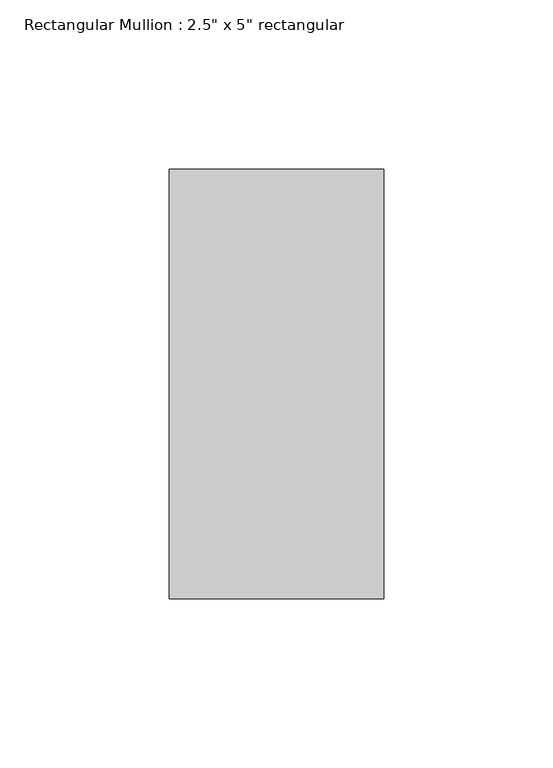
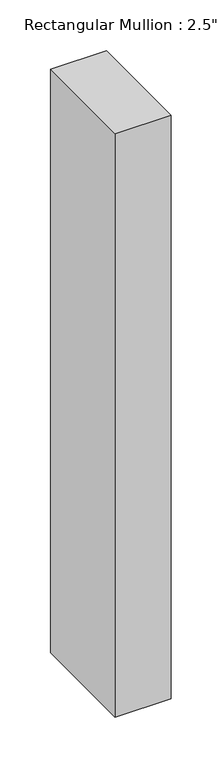
"""IFC4 building model written with IfcOpenShell, lengths in millimetres: member geometry."""

from ifc_helpers import new_model, si_unit, frame, origin, place, context, project, spatial, polyline, outline, extrude, source, transform, mapped, element, save


def member_94a221ea(model_context):
    return source(origin(), model_context, "Body", "SweptSolid", [
        extrude(outline(polyline([(0.0, 63.5), (0.0, -63.5), (-63.5, -63.5), (-63.5, 63.5), (0.0, 63.5)])), frame((0.0, 0.0, -700.6166667), z_axis=(0.0, 0.0, 1.0), x_axis=(1.0, 0.0, 0.0)), (0.0, 0.0, 1.0), 700.6166667),
    ])


if __name__ == "__main__":
    model = new_model("IFC4")
    model_context = context("Model", 3, world=origin())
    ifc_project = project(units=[si_unit("LENGTHUNIT", "METRE", prefix="MILLI")], contexts=[model_context])
    site = spatial("IfcSite", under=ifc_project)
    building = spatial("IfcBuilding", under=site)
    placement = place(None, origin())
    member_shape = member_94a221ea(model_context)
    element("IfcMember", 1, ObjectType="Rectangular Mullion : 2.5\" x 5\" rectangular", at=placement, inside=building, context=model_context, shape_type="MappedRepresentation", body=[
        mapped(member_shape, transform((0.0, 0.0, 0.0), x_axis=(1.0, 0.0, 0.0), y_axis=(0.0, 1.0, 0.0), z_axis=(0.0, 0.0, 1.0))),
    ])
    save(model, "model.ifc")

# Revit data of these elements
# Type "Rectangular Mullion : 2.5\" x 5\" rectangular"
#   built-in parameter 1007304 = 0.416667 (stored number, unit not read)
#   built-in parameter 1007301 = 0.104167 (stored number, unit not read)
#   built-in parameter 1007300 = 0.104167 (stored number, unit not read)
# Element 1 (IfcMember, "Rectangular Mullion : 2.5\" x 5\" rectangular")
#   Materials on its faces: "Aluminum"
# Materials
#   "Aluminum": class "Metal", colour RGB 247 247 247, transparency 0, Description = "Aluminum 6061", Cost = 0
